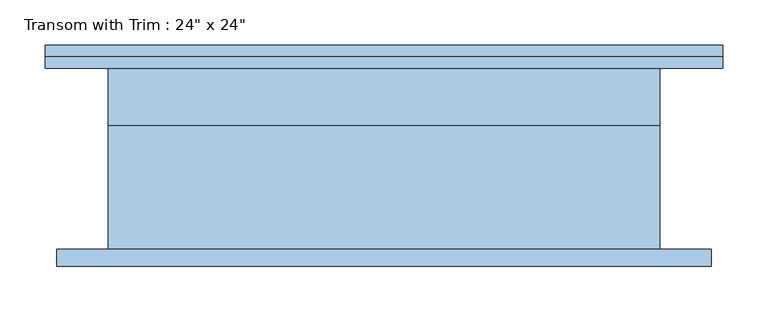
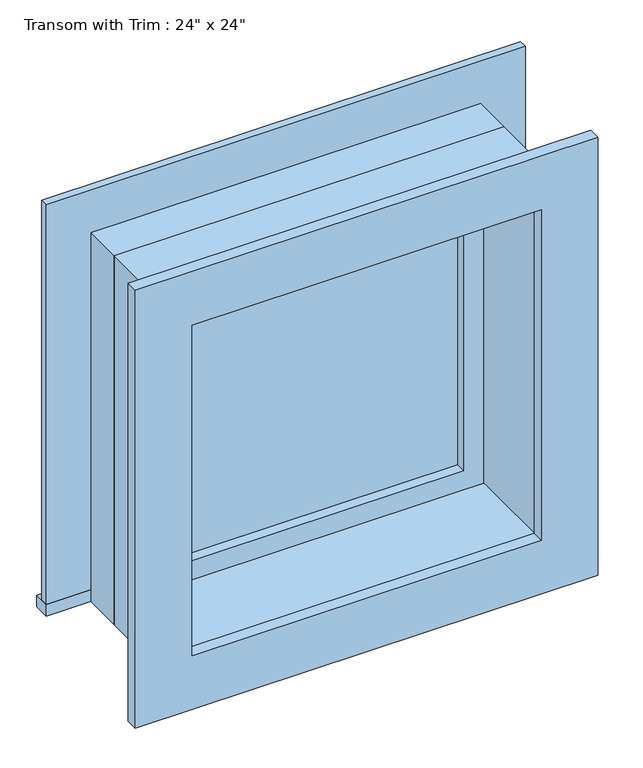
"""IFC4 building model written with IfcOpenShell, lengths in millimetres: window geometry."""

from ifc_helpers import new_model, si_unit, frame, origin, place, context, project, spatial, polyline, outline, extrude, source, transform, mapped, element, save


def window_1a9eb5ca(model_context):
    return source(origin(), model_context, "Body", "SweptSolid", [
        extrude(outline(polyline([(-412.75, 125.4), (336.55, 125.4), (336.55, 100.0), (-412.75, 100.0), (-412.75, 125.4)])), frame((0.0, 0.0, 2159.0), z_axis=(0.0, 0.0, 1.0), x_axis=(1.0, 0.0, 0.0)), (0.0, 0.0, 1.0), 19.05),
        extrude(outline(polyline([(2749.55, -323.85), (2749.55, 247.65), (2178.05, 247.65), (2178.05, 336.55), (2838.45, 336.55), (2838.45, -412.75), (2178.05, -412.75), (2178.05, -323.85), (2749.55, -323.85)])), frame((0.0, 100.0, 0.0), z_axis=(0.0, 1.0, 0.0), x_axis=(0.0, 0.0, 1.0)), (0.0, 0.0, 1.0), 12.7),
        extrude(outline(polyline([(2825.75, 323.85), (2825.75, -400.05), (2101.85, -400.05), (2101.85, 323.85), (2825.75, 323.85)]), holes=[polyline([(2736.85, 234.95), (2190.75, 234.95), (2190.75, -311.15), (2736.85, -311.15), (2736.85, 234.95)])]), frame((0.0, -119.05, 0.0), z_axis=(0.0, 1.0, 0.0), x_axis=(0.0, 0.0, 1.0)), (0.0, 0.0, 1.0), 19.05),
        extrude(outline(polyline([(203.2, 52.375), (-279.4, 52.375), (-279.4, 65.075), (203.2, 65.075), (203.2, 52.375)])), frame((0.0, 0.0, 2222.5), z_axis=(0.0, 0.0, 1.0), x_axis=(1.0, 0.0, 0.0)), (0.0, 0.0, 1.0), 482.6),
        extrude(outline(polyline([(2749.55, -323.85), (2178.05, -323.85), (2178.05, 247.65), (2749.55, 247.65), (2749.55, -323.85)]), holes=[polyline([(2705.1, -279.4), (2705.1, 203.2), (2222.5, 203.2), (2222.5, -279.4), (2705.1, -279.4)])]), frame((0.0, 36.5, 0.0), z_axis=(0.0, 1.0, 0.0), x_axis=(0.0, 0.0, 1.0)), (0.0, 0.0, 1.0), 44.45),
        extrude(outline(polyline([(2768.6, -342.9), (2159.0, -342.9), (2159.0, 266.7), (2768.6, 266.7), (2768.6, -342.9)]), holes=[polyline([(2736.85, -311.15), (2736.85, 234.95), (2190.75, 234.95), (2190.75, -311.15), (2736.85, -311.15)])]), frame((0.0, -100.0, 0.0), z_axis=(0.0, 1.0, 0.0), x_axis=(0.0, 0.0, 1.0)), (0.0, 0.0, 1.0), 136.5),
        extrude(outline(polyline([(2768.6, 266.7), (2768.6, -342.9), (2159.0, -342.9), (2159.0, 266.7), (2768.6, 266.7)]), holes=[polyline([(2749.55, 247.65), (2178.05, 247.65), (2178.05, -323.85), (2749.55, -323.85), (2749.55, 247.65)])]), frame((0.0, 36.5, 0.0), z_axis=(0.0, 1.0, 0.0), x_axis=(0.0, 0.0, 1.0)), (0.0, 0.0, 1.0), 63.5),
    ])


if __name__ == "__main__":
    model = new_model("IFC4")
    model_context = context("Model", 3, world=origin())
    ifc_project = project(units=[si_unit("LENGTHUNIT", "METRE", prefix="MILLI")], contexts=[model_context])
    site = spatial("IfcSite", under=ifc_project)
    building = spatial("IfcBuilding", under=site)
    placement = place(None, origin())
    window_shape = window_1a9eb5ca(model_context)
    element("IfcWindow", 1, ObjectType="Transom with Trim : 24\" x 24\"", at=placement, inside=building, context=model_context, shape_type="MappedRepresentation", body=[
        mapped(window_shape, transform((0.0, 0.0, 0.0), x_axis=(1.0, 0.0, 0.0), y_axis=(0.0, 1.0, 0.0), z_axis=(0.0, 0.0, 1.0))),
    ])
    save(model, "model.ifc")

# Revit data of these elements
# Type "Transom with Trim : 24\" x 24\""
#   Type Mark = "22"
#   Construction Type Id = "GSP4R"
#   Assembly Code = "B2020100"
#   Analytic Construction = "1/8 in Pilkington single glazing"
#   Visual Light Transmittance = 0.9
#   Solar Heat Gain Coefficient = 0.78
#   Heat Transfer Coefficient (U) = 3.6886 W/(m²·K)
#   Height = 2' - 0"
#   Default Sill Height = 7' - 1"
#   Trim Projection - Ext. = 0' - 0 1/2"
#   Trim Projection - Int. = 0' - 0 3/4"
#   Trim Width - Exterior = 0' - 3 1/2"
#   Trim Width - Interior = 0' - 3 1/2"
#   Width = 2' - 0"
#   Window Inset = 0' - 0 3/4"
#   Define Thermal Properties by = 1
#   Glass Pane Material = Glass
#   Sash Material = Sash
#   Trim Exterior Material = Trim
#   Trim Interior Material = Trim
#   Wall Closure = (empty or 0)
# Element 1 (IfcWindow, "Transom with Trim : 24\" x 24\"")
#   Materials on its faces: "Sash", "Trim", "Glass"
# Materials
#   "Glass": class "Glass", colour RGB 218 227 224, transparency 0.85, Description = "Soda Lime Glass", Cost = 0
#   "Sash": class "Wood", colour RGB 136 99 55, transparency 0
#   "Trim": class "Wood", colour RGB 224 178 126, transparency 0
